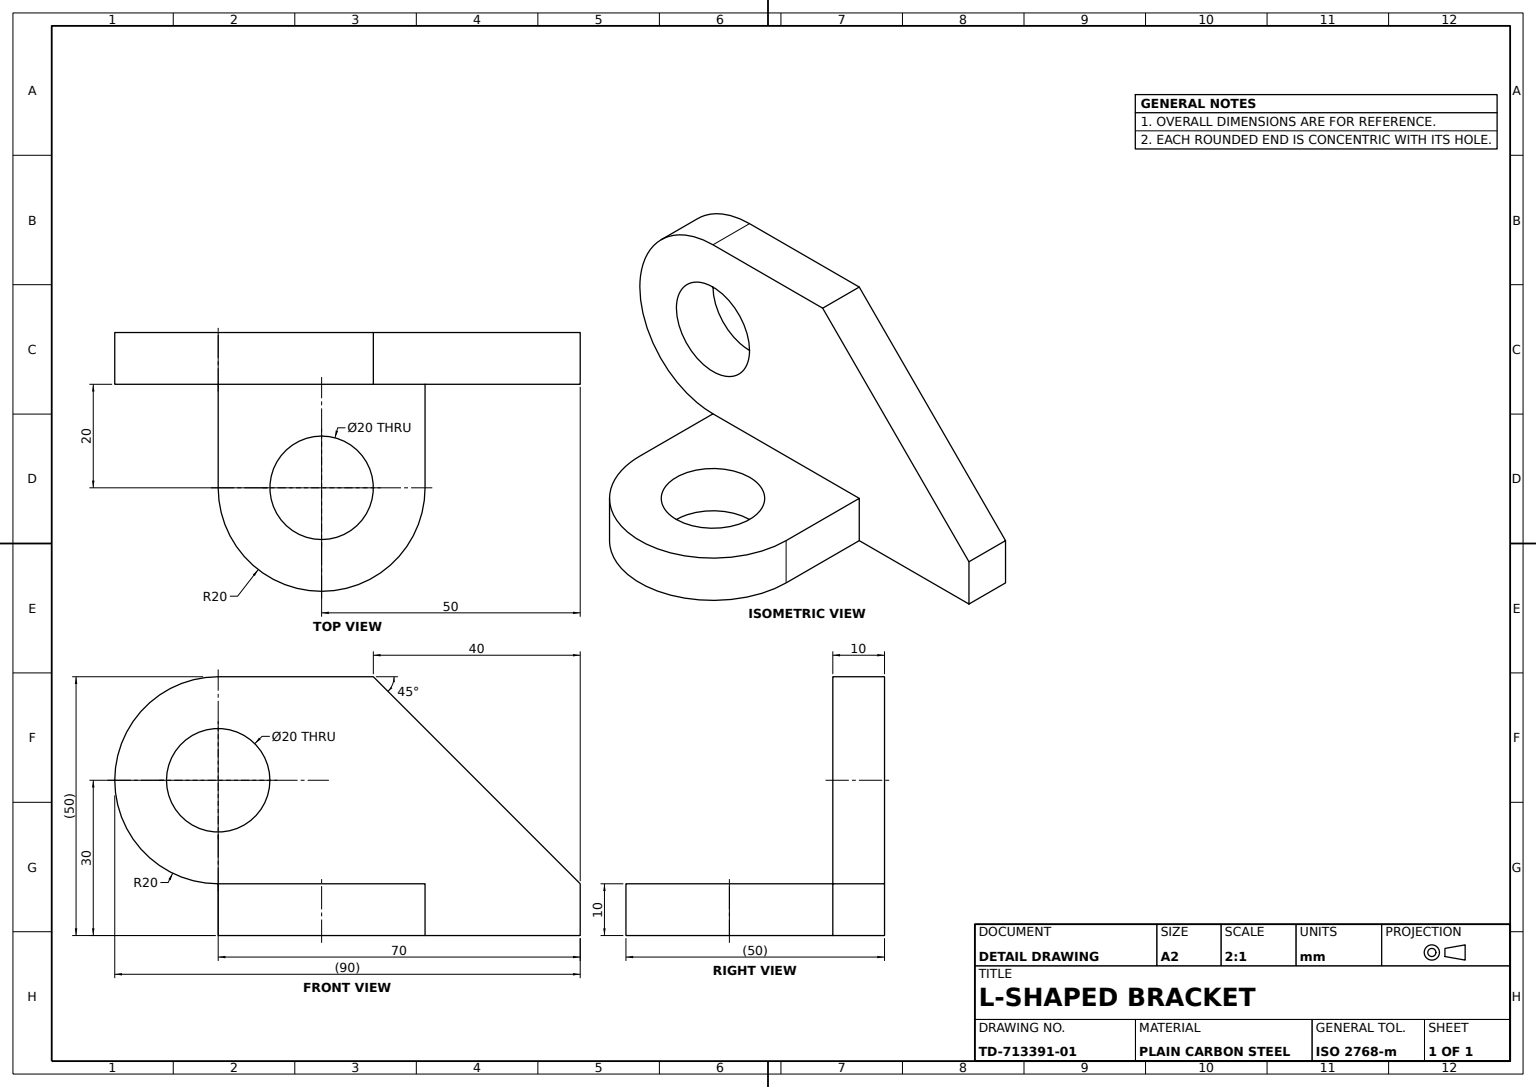
from build123d import *

# Parameters (mm, degrees)
UPRIGHT_PLATE_DEPTH          = 5
BASE_LUG_DEPTH               = 10
BASE_LUG_HOLE_PROFILE_R      = 10
BASE_LUG_HOLE_20_DEPTH       = 93.330926563
UPRIGHT_PLATE_HOLE_PROFILE_R = 10
UPRIGHT_PLATE_HOLE_20_DEPTH  = 95.868329805


with BuildPart() as part:
    # Upright Plate Profile → Upright Plate (new, symmetric)
    with BuildSketch(Plane.XY):
        with BuildLine():
            Line((0, 50), (30, 50))
            Line((30, 50), (70, 10))
            Line((70, 10), (70, 0))
            Line((70, 0), (0, 0))
            Line((0, 0), (0, 10))
            ThreePointArc((0, 10), (-20, 30), (0, 50))
        make_face()
    extrude(amount=UPRIGHT_PLATE_DEPTH, both=True)

    # Base Lug Profile → Base Lug (add)
    with BuildSketch(Plane.XZ):
        with BuildLine():
            Line((0, 5), (0, 25))
            ThreePointArc((0, 25), (20, 45), (40, 25))
            Line((40, 25), (40, 5))
            Line((40, 5), (70, 5))
            Line((70, 5), (70, -5))
            Line((70, -5), (0, -5))
            Line((0, -5), (0, 5))
        make_face()
    extrude(amount=-BASE_LUG_DEPTH)

    # Base Lug Hole Profile → Base Lug Hole Ø20 (cut, through all)
    with BuildSketch(Plane(origin=(0, 10, 0), x_dir=(1, 0, 0), z_dir=(0, 1, 0))):
        with Locations(Location((20, -25, 0), (0, 0, 270))):
            Circle(BASE_LUG_HOLE_PROFILE_R)
    extrude(amount=-BASE_LUG_HOLE_20_DEPTH, mode=Mode.SUBTRACT)

    # Upright Plate Hole Profile → Upright Plate Hole Ø20 (cut, through all)
    with BuildSketch(Plane.XY.offset(5)):
        with Locations((0, 30)):
            Circle(UPRIGHT_PLATE_HOLE_PROFILE_R)
    extrude(amount=-UPRIGHT_PLATE_HOLE_20_DEPTH, mode=Mode.SUBTRACT)


solid = part.part
